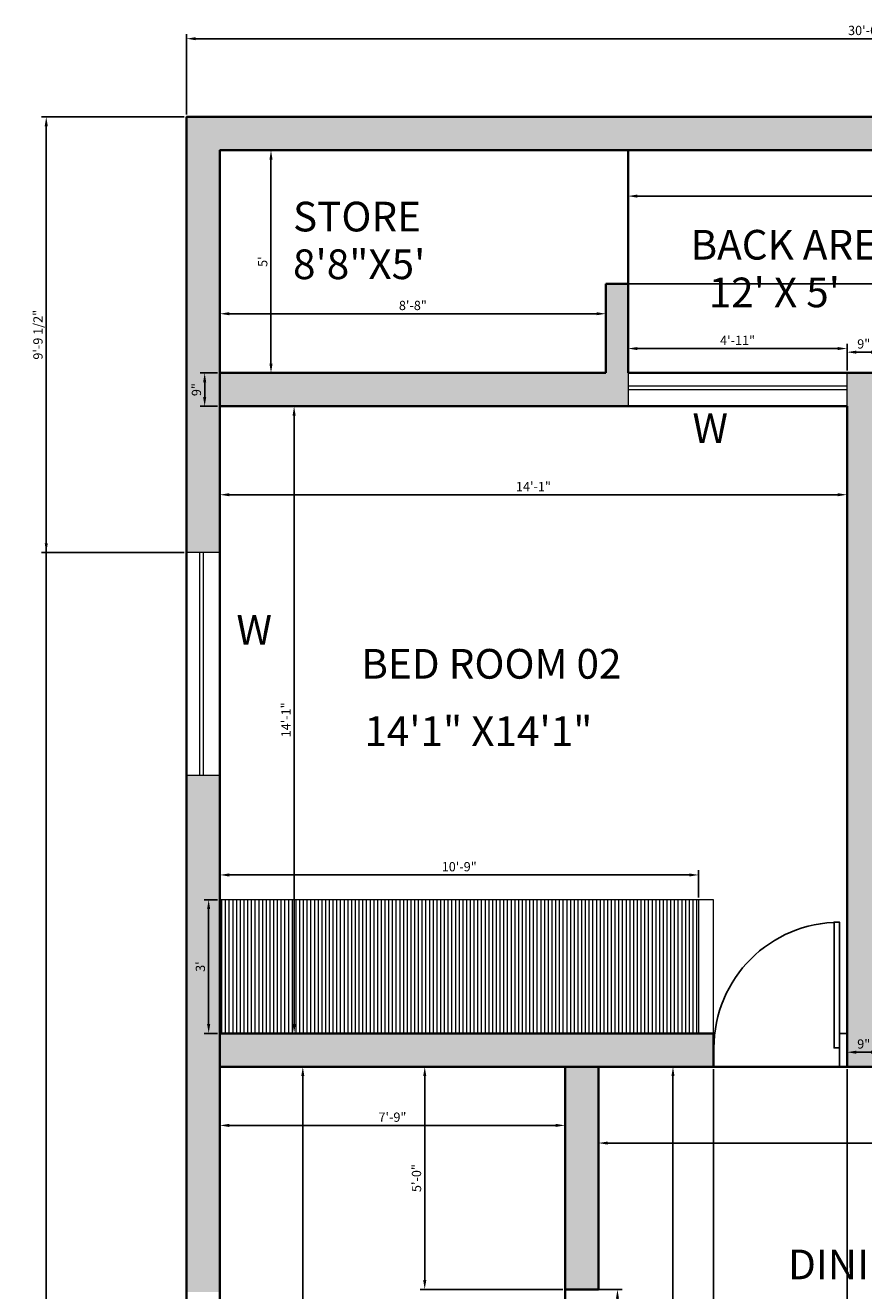
# Model space of a CAD drawing. Units: inches. Extents: x 844 to 1293, y 1224 to 2014.
# Tile 3 of 4: x 844 to 1070, y 1673 to 2014. Entities that reach past the tile are written whole.
import ezdxf

# ---------------------------------------------------------------- set-up
doc = ezdxf.new("R2010")
doc.units = ezdxf.units.IN
for name, color, linetype, lineweight in [('A-ANNO-DIMS', 2, 'Continuous', 18), ('A-ANNO-TEXT', 3, 'Continuous', 18), ('A-AREA-IDEN', 7, 'Continuous', 25), ('A-DOOR', 3, 'Continuous', 25), ('A-FLOR-PATT', 8, 'Continuous', 13), ('A-GLAZ', 4, 'Continuous', 18), ('A-WALL', 7, 'Continuous', 35), ('A-WALL-PATT', 252, 'Continuous', 13)]:
    doc.layers.add(name, color=color, linetype=linetype, lineweight=lineweight)
doc.styles.get("Standard").update_dxf_attribs({"font": 'arial.ttf'})
doc.dimstyles.new('Copy of ISO-25', dxfattribs={"dimtxt": 2.5, "dimasz": 2.5, "dimexe": 1.25, "dimexo": 0.625, "dimtad": 1, "dimlunit": 4, "dimtxsty": 'Standard', "dimcen": 2.5, "dimadec": 0, "dimazin": 0, "dimtfac": 1, "dimtmove": 0, "dimatfit": 3, "dimfxl": 1, "dimarcsym": 0})

# ---------------------------------------------------------------- blocks, each defined once
blk = doc.blocks.new('*U2')
for p, q in [((0, 0), (0, -6)), ((-40, 0), (-40, -6))]:
    blk.add_line(p, q)
blk.add_lwpolyline([(0, 0), (0, 40), (-1.75, 40), (-1.75, 0)], close=True)
blk.add_arc((0, 0), 40, 90, 180)
blk = doc.blocks.new('*D7')
at = {"layer": 'A-ANNO-DIMS', "color": 0, "lineweight": -2, "transparency": 16777216}
for p, q in [((896.46, 1910.42), (896.46, 1885.96)), ((1065.46, 1910.42), (1065.46, 1885.96)), ((898.96, 1887.21), (1062.96, 1887.21))]:
    blk.add_line(p, q, dxfattribs=at)
at = {"layer": 'A-ANNO-DIMS', "color": 0, "transparency": 16777216}
for points in [[(898.96, 1887.63), (898.96, 1886.8), (896.46, 1887.21)], [(1062.96, 1887.63), (1062.96, 1886.8), (1065.46, 1887.21)]]:
    blk.add_solid(points, dxfattribs=at)
at = {"layer": 'Defpoints', "color": 0, "transparency": 16777216}
for p in [(896.46, 1911.04), (1065.46, 1911.04), (1065.46, 1887.21)]:
    blk.add_point(p, dxfattribs=at)
at = {"layer": 'A-ANNO-DIMS', "color": 0, "transparency": 16777216, "insert": (980.96, 1889.09), "char_height": 2.5, "attachment_point": 5}
blk.add_mtext('14\'-1"', dxfattribs=at)
blk = doc.blocks.new('*D8')
at = {"layer": 'A-ANNO-DIMS', "color": 0, "lineweight": -2, "transparency": 16777216}
for p, q in [((897.09, 1911.04), (917.71, 1911.04)), ((916.46, 1908.54), (916.46, 1744.54)), ((897.09, 1742.04), (917.71, 1742.04))]:
    blk.add_line(p, q, dxfattribs=at)
at = {"layer": 'A-ANNO-DIMS', "color": 0, "transparency": 16777216}
for points in [[(916.05, 1908.54), (916.88, 1908.54), (916.46, 1911.04)], [(916.05, 1744.54), (916.88, 1744.54), (916.46, 1742.04)]]:
    blk.add_solid(points, dxfattribs=at)
at = {"layer": 'Defpoints', "color": 0, "transparency": 16777216}
for p in [(896.46, 1911.04), (896.46, 1742.04), (916.46, 1742.04)]:
    blk.add_point(p, dxfattribs=at)
at = {"layer": 'A-ANNO-DIMS', "color": 0, "transparency": 16777216, "insert": (914.58, 1826.54), "char_height": 2.5, "attachment_point": 5, "rotation": 90}
blk.add_mtext('14\'-1"', dxfattribs=at)
blk = doc.blocks.new('*D9')
at = {"layer": 'A-ANNO-DIMS', "color": 0, "lineweight": -2, "transparency": 16777216}
for p, q in [((896.46, 1920.67), (896.46, 1937.24)), ((1000.46, 1920.67), (1000.46, 1937.24)), ((898.96, 1935.99), (997.96, 1935.99))]:
    blk.add_line(p, q, dxfattribs=at)
at = {"layer": 'A-ANNO-DIMS', "color": 0, "transparency": 16777216}
for points in [[(898.96, 1936.41), (898.96, 1935.58), (896.46, 1935.99)], [(997.96, 1936.41), (997.96, 1935.58), (1000.46, 1935.99)]]:
    blk.add_solid(points, dxfattribs=at)
at = {"layer": 'Defpoints', "color": 0, "transparency": 16777216}
for p in [(1000.46, 1935.99), (896.46, 1920.04), (1000.46, 1920.04)]:
    blk.add_point(p, dxfattribs=at)
at = {"layer": 'A-ANNO-DIMS', "color": 0, "transparency": 16777216, "insert": (948.46, 1937.9), "char_height": 2.5, "attachment_point": 5}
blk.add_mtext('8\'-8"', dxfattribs=at)
blk = doc.blocks.new('*D10')
at = {"layer": 'A-ANNO-DIMS', "color": 0, "lineweight": -2, "transparency": 16777216}
for p, q in [((897.09, 1980.04), (911.48, 1980.04)), ((910.23, 1977.54), (910.23, 1922.54)), ((897.09, 1920.04), (911.48, 1920.04))]:
    blk.add_line(p, q, dxfattribs=at)
at = {"layer": 'A-ANNO-DIMS', "color": 0, "transparency": 16777216}
for points in [[(909.81, 1977.54), (910.65, 1977.54), (910.23, 1980.04)], [(909.81, 1922.54), (910.65, 1922.54), (910.23, 1920.04)]]:
    blk.add_solid(points, dxfattribs=at)
at = {"layer": 'Defpoints', "color": 0, "transparency": 16777216}
for p in [(896.46, 1980.04), (896.46, 1920.04), (910.23, 1920.04)]:
    blk.add_point(p, dxfattribs=at)
at = {"layer": 'A-ANNO-DIMS', "color": 0, "transparency": 16777216, "insert": (908.33, 1950.04), "char_height": 2.5, "attachment_point": 5, "rotation": 90}
blk.add_mtext("5'", dxfattribs=at)
blk = doc.blocks.new('*D11')
at = {"layer": 'A-ANNO-DIMS', "color": 0, "lineweight": -2, "transparency": 16777216}
for p, q in [((1006.46, 1979.42), (1006.46, 1966.44)), ((1150.46, 1979.42), (1150.46, 1966.44)), ((1008.96, 1967.69), (1147.96, 1967.69))]:
    blk.add_line(p, q, dxfattribs=at)
at = {"layer": 'A-ANNO-DIMS', "color": 0, "transparency": 16777216}
for points in [[(1008.96, 1968.11), (1008.96, 1967.27), (1006.46, 1967.69)], [(1147.96, 1968.11), (1147.96, 1967.27), (1150.46, 1967.69)]]:
    blk.add_solid(points, dxfattribs=at)
at = {"layer": 'Defpoints', "color": 0, "transparency": 16777216}
for p in [(1006.46, 1980.04), (1150.46, 1980.04), (1150.46, 1967.69)]:
    blk.add_point(p, dxfattribs=at)
at = {"layer": 'A-ANNO-DIMS', "color": 0, "transparency": 16777216, "insert": (1078.46, 1969.57), "char_height": 2.5, "attachment_point": 5}
blk.add_mtext("12'", dxfattribs=at)
blk = doc.blocks.new('*D15')
at = {"layer": 'A-ANNO-DIMS', "color": 0, "lineweight": -2, "transparency": 16777216}
for p, q in [((896.46, 1732.42), (896.46, 1715.99)), ((989.46, 1732.42), (989.46, 1715.99)), ((898.96, 1717.24), (986.96, 1717.24))]:
    blk.add_line(p, q, dxfattribs=at)
at = {"layer": 'A-ANNO-DIMS', "color": 0, "transparency": 16777216}
for points in [[(898.96, 1717.66), (898.96, 1716.82), (896.46, 1717.24)], [(986.96, 1717.66), (986.96, 1716.82), (989.46, 1717.24)]]:
    blk.add_solid(points, dxfattribs=at)
at = {"layer": 'Defpoints', "color": 0, "transparency": 16777216}
for p in [(896.46, 1733.04), (989.46, 1733.04), (989.46, 1717.24)]:
    blk.add_point(p, dxfattribs=at)
at = {"layer": 'A-ANNO-DIMS', "color": 0, "transparency": 16777216, "insert": (942.96, 1719.14), "char_height": 2.5, "attachment_point": 5}
blk.add_mtext('7\'-9"', dxfattribs=at)
blk = doc.blocks.new('*D16')
at = {"layer": 'A-ANNO-DIMS', "color": 0, "lineweight": -2, "transparency": 16777216}
for p, q in [((897.09, 1733.04), (920.05, 1733.04)), ((918.8, 1730.54), (918.8, 1565.54)), ((897.09, 1563.04), (920.05, 1563.04))]:
    blk.add_line(p, q, dxfattribs=at)
at = {"layer": 'A-ANNO-DIMS', "color": 0, "transparency": 16777216}
for points in [[(918.39, 1730.54), (919.22, 1730.54), (918.8, 1733.04)], [(918.39, 1565.54), (919.22, 1565.54), (918.8, 1563.04)]]:
    blk.add_solid(points, dxfattribs=at)
at = {"layer": 'Defpoints', "color": 0, "transparency": 16777216}
for p in [(896.46, 1733.04), (896.46, 1563.04), (918.8, 1563.04)]:
    blk.add_point(p, dxfattribs=at)
at = {"layer": 'A-ANNO-DIMS', "color": 0, "transparency": 16777216, "insert": (916.92, 1648.04), "char_height": 2.5, "attachment_point": 5, "rotation": 90}
blk.add_mtext('14\'-2"', dxfattribs=at)
blk = doc.blocks.new('*D18')
at = {"layer": 'A-ANNO-DIMS', "color": 0, "lineweight": -2, "transparency": 16777216}
for p, q in [((998.46, 1732.42), (998.46, 1711.23)), ((1244.46, 1732.42), (1244.46, 1711.23)), ((1000.96, 1712.48), (1241.96, 1712.48))]:
    blk.add_line(p, q, dxfattribs=at)
at = {"layer": 'A-ANNO-DIMS', "color": 0, "transparency": 16777216}
for points in [[(1000.96, 1712.89), (1000.96, 1712.06), (998.46, 1712.48)], [(1241.96, 1712.89), (1241.96, 1712.06), (1244.46, 1712.48)]]:
    blk.add_solid(points, dxfattribs=at)
at = {"layer": 'Defpoints', "color": 0, "transparency": 16777216}
for p in [(998.46, 1733.04), (1244.46, 1733.04), (1244.46, 1712.48)]:
    blk.add_point(p, dxfattribs=at)
at = {"layer": 'A-ANNO-DIMS', "color": 0, "transparency": 16777216, "insert": (1121.46, 1714.38), "char_height": 2.5, "attachment_point": 5}
blk.add_mtext('20\'-6"', dxfattribs=at)
blk = doc.blocks.new('*D19')
at = {"layer": 'A-ANNO-DIMS', "color": 0, "lineweight": -2, "transparency": 16777216}
for p, q in [((999.09, 1733.04), (1019.81, 1733.04)), ((1018.56, 1730.54), (1018.56, 1556.54)), ((999.09, 1554.04), (1019.81, 1554.04))]:
    blk.add_line(p, q, dxfattribs=at)
at = {"layer": 'A-ANNO-DIMS', "color": 0, "transparency": 16777216}
for points in [[(1018.14, 1730.54), (1018.97, 1730.54), (1018.56, 1733.04)], [(1018.14, 1556.54), (1018.97, 1556.54), (1018.56, 1554.04)]]:
    blk.add_solid(points, dxfattribs=at)
at = {"layer": 'Defpoints', "color": 0, "transparency": 16777216}
for p in [(998.46, 1733.04), (998.46, 1554.04), (1018.56, 1554.04)]:
    blk.add_point(p, dxfattribs=at)
at = {"layer": 'A-ANNO-DIMS', "color": 0, "transparency": 16777216, "insert": (1016.68, 1643.54), "char_height": 2.5, "attachment_point": 5, "rotation": 90}
blk.add_mtext('14\'-11"', dxfattribs=at)
blk = doc.blocks.new('*D26')
at = {"layer": 'A-ANNO-DIMS', "color": 0, "lineweight": -2, "transparency": 16777216}
for p, q in [((1006.46, 1920.67), (1006.46, 1927.86)), ((1065.46, 1920.67), (1065.46, 1927.86)), ((1008.96, 1926.61), (1062.96, 1926.61))]:
    blk.add_line(p, q, dxfattribs=at)
at = {"layer": 'A-ANNO-DIMS', "color": 0, "transparency": 16777216}
for points in [[(1008.96, 1927.02), (1008.96, 1926.19), (1006.46, 1926.61)], [(1062.96, 1927.02), (1062.96, 1926.19), (1065.46, 1926.61)]]:
    blk.add_solid(points, dxfattribs=at)
at = {"layer": 'Defpoints', "color": 0, "transparency": 16777216}
for p in [(1065.46, 1926.61), (1006.46, 1920.04), (1065.46, 1920.04)]:
    blk.add_point(p, dxfattribs=at)
at = {"layer": 'A-ANNO-DIMS', "color": 0, "transparency": 16777216, "insert": (1035.96, 1928.49), "char_height": 2.5, "attachment_point": 5}
blk.add_mtext('4\'-11"', dxfattribs=at)
blk = doc.blocks.new('*D30')
at = {"layer": 'A-ANNO-DIMS', "color": 0, "lineweight": -2, "transparency": 16777216}
for p, q in [((887.46, 1989.67), (887.46, 2011.37)), ((889.96, 2010.12), (1250.96, 2010.12)), ((1253.46, 1989.67), (1253.46, 2011.37))]:
    blk.add_line(p, q, dxfattribs=at)
at = {"layer": 'A-ANNO-DIMS', "color": 0, "transparency": 16777216}
for points in [[(889.96, 2010.54), (889.96, 2009.71), (887.46, 2010.12)], [(1250.96, 2010.54), (1250.96, 2009.71), (1253.46, 2010.12)]]:
    blk.add_solid(points, dxfattribs=at)
at = {"layer": 'Defpoints', "color": 0, "transparency": 16777216}
for p in [(1253.46, 2010.12), (887.46, 1989.04), (1253.46, 1989.04)]:
    blk.add_point(p, dxfattribs=at)
at = {"layer": 'A-ANNO-DIMS', "color": 0, "transparency": 16777216, "insert": (1070.46, 2012.02), "char_height": 2.5, "attachment_point": 5}
blk.add_mtext('30\'-6"', dxfattribs=at)
blk = doc.blocks.new('*D34')
at = {"layer": 'A-ANNO-DIMS', "color": 0, "lineweight": -2, "transparency": 16777216}
for p, q in [((1065.46, 1920.67), (1065.46, 1926.88)), ((1074.46, 1920.67), (1074.46, 1926.88)), ((1067.96, 1925.63), (1071.96, 1925.63))]:
    blk.add_line(p, q, dxfattribs=at)
at = {"layer": 'A-ANNO-DIMS', "color": 0, "transparency": 16777216}
for points in [[(1067.96, 1926.05), (1067.96, 1925.22), (1065.46, 1925.63)], [(1071.96, 1926.05), (1071.96, 1925.22), (1074.46, 1925.63)]]:
    blk.add_solid(points, dxfattribs=at)
at = {"layer": 'Defpoints', "color": 0, "transparency": 16777216}
for p in [(1074.46, 1925.63), (1065.46, 1920.04), (1074.46, 1920.04)]:
    blk.add_point(p, dxfattribs=at)
at = {"layer": 'A-ANNO-DIMS', "color": 0, "transparency": 16777216, "insert": (1069.96, 1927.53), "char_height": 2.5, "attachment_point": 5}
blk.add_mtext('9"', dxfattribs=at)
blk = doc.blocks.new('*D35')
at = {"layer": 'A-ANNO-DIMS', "color": 0, "lineweight": -2, "transparency": 16777216}
for p, q in [((895.84, 1920.04), (891.11, 1920.04)), ((892.36, 1913.54), (892.36, 1917.54)), ((895.84, 1911.04), (891.11, 1911.04))]:
    blk.add_line(p, q, dxfattribs=at)
at = {"layer": 'A-ANNO-DIMS', "color": 0, "transparency": 16777216}
for points in [[(891.94, 1917.54), (892.77, 1917.54), (892.36, 1920.04)], [(891.94, 1913.54), (892.77, 1913.54), (892.36, 1911.04)]]:
    blk.add_solid(points, dxfattribs=at)
at = {"layer": 'Defpoints', "color": 0, "transparency": 16777216}
for p in [(892.36, 1920.04), (896.46, 1920.04), (896.46, 1911.04)]:
    blk.add_point(p, dxfattribs=at)
at = {"layer": 'A-ANNO-DIMS', "color": 0, "transparency": 16777216, "insert": (890.45, 1915.54), "char_height": 2.5, "attachment_point": 5, "rotation": 90}
blk.add_mtext('9"', dxfattribs=at)
blk = doc.blocks.new('*D36')
at = {"layer": 'A-ANNO-DIMS', "color": 0, "lineweight": -2, "transparency": 16777216}
for p, q in [((1065.46, 1733.67), (1065.46, 1738.21)), ((1067.96, 1736.96), (1071.96, 1736.96)), ((1074.46, 1733.67), (1074.46, 1738.21))]:
    blk.add_line(p, q, dxfattribs=at)
at = {"layer": 'A-ANNO-DIMS', "color": 0, "transparency": 16777216}
for points in [[(1067.96, 1737.38), (1067.96, 1736.54), (1065.46, 1736.96)], [(1071.96, 1737.38), (1071.96, 1736.54), (1074.46, 1736.96)]]:
    blk.add_solid(points, dxfattribs=at)
at = {"layer": 'Defpoints', "color": 0, "transparency": 16777216}
for p in [(1074.46, 1736.96), (1065.46, 1733.04), (1074.46, 1733.04)]:
    blk.add_point(p, dxfattribs=at)
at = {"layer": 'A-ANNO-DIMS', "color": 0, "transparency": 16777216, "insert": (1069.96, 1738.86), "char_height": 2.5, "attachment_point": 5}
blk.add_mtext('9"', dxfattribs=at)
blk = doc.blocks.new('*D39')
at = {"layer": 'A-ANNO-DIMS', "color": 0, "lineweight": -2, "transparency": 16777216}
for p, q in [((895.84, 1778.04), (892.18, 1778.04)), ((893.43, 1775.54), (893.43, 1744.54)), ((895.84, 1742.04), (892.18, 1742.04))]:
    blk.add_line(p, q, dxfattribs=at)
at = {"layer": 'A-ANNO-DIMS', "color": 0, "transparency": 16777216}
for points in [[(893.01, 1775.54), (893.84, 1775.54), (893.43, 1778.04)], [(893.01, 1744.54), (893.84, 1744.54), (893.43, 1742.04)]]:
    blk.add_solid(points, dxfattribs=at)
at = {"layer": 'Defpoints', "color": 0, "transparency": 16777216}
for p in [(896.46, 1778.04), (893.43, 1742.04), (896.46, 1742.04)]:
    blk.add_point(p, dxfattribs=at)
at = {"layer": 'A-ANNO-DIMS', "color": 0, "transparency": 16777216, "insert": (891.52, 1760.04), "char_height": 2.5, "attachment_point": 5, "rotation": 90}
blk.add_mtext("3'", dxfattribs=at)
blk = doc.blocks.new('*D40')
at = {"layer": 'A-ANNO-DIMS', "color": 0, "lineweight": -2, "transparency": 16777216}
for p, q in [((896.46, 1778.67), (896.46, 1785.99)), ((898.96, 1784.74), (1022.96, 1784.74)), ((1025.46, 1778.67), (1025.46, 1785.99))]:
    blk.add_line(p, q, dxfattribs=at)
at = {"layer": 'A-ANNO-DIMS', "color": 0, "transparency": 16777216}
for points in [[(898.96, 1785.15), (898.96, 1784.32), (896.46, 1784.74)], [(1022.96, 1785.15), (1022.96, 1784.32), (1025.46, 1784.74)]]:
    blk.add_solid(points, dxfattribs=at)
at = {"layer": 'Defpoints', "color": 0, "transparency": 16777216}
for p in [(1025.46, 1784.74), (896.46, 1778.04), (1025.46, 1778.04)]:
    blk.add_point(p, dxfattribs=at)
at = {"layer": 'A-ANNO-DIMS', "color": 0, "transparency": 16777216, "insert": (960.96, 1786.64), "char_height": 2.5, "attachment_point": 5}
blk.add_mtext('10\'-9"', dxfattribs=at)
blk = doc.blocks.new('*D42')
at = {"layer": 'A-ANNO-DIMS', "color": 0, "lineweight": -2, "transparency": 16777216}
for p, q in [((990.09, 1673.04), (1004.85, 1673.04)), ((1003.6, 1625.54), (1003.6, 1670.54)), ((990.09, 1623.04), (1004.85, 1623.04))]:
    blk.add_line(p, q, dxfattribs=at)
at = {"layer": 'A-ANNO-DIMS', "color": 0, "transparency": 16777216}
for points in [[(1003.19, 1670.54), (1004.02, 1670.54), (1003.6, 1673.04)], [(1003.19, 1625.54), (1004.02, 1625.54), (1003.6, 1623.04)]]:
    blk.add_solid(points, dxfattribs=at)
at = {"layer": 'Defpoints', "color": 0, "transparency": 16777216}
for p in [(989.46, 1673.04), (1003.6, 1673.04), (989.46, 1623.04)]:
    blk.add_point(p, dxfattribs=at)
at = {"layer": 'A-ANNO-DIMS', "color": 0, "transparency": 16777216, "insert": (1001.72, 1648.04), "char_height": 2.5, "attachment_point": 5, "rotation": 90}
blk.add_mtext('4\'-2"', dxfattribs=at)
blk = doc.blocks.new('WIN-GLAZ-60IN')
for p, q in [((0, 60), (0, 0)), ((1, 60), (1, 0))]:
    blk.add_line(p, q)
blk = doc.blocks.new('*D51')
at = {"layer": 'A-ANNO-DIMS', "color": 0, "lineweight": -2, "transparency": 16777216}
for p, q in [((988.84, 1733.04), (950.41, 1733.04)), ((951.66, 1675.54), (951.66, 1730.54)), ((988.84, 1673.04), (950.41, 1673.04))]:
    blk.add_line(p, q, dxfattribs=at)
at = {"layer": 'A-ANNO-DIMS', "color": 0, "transparency": 16777216}
for points in [[(951.25, 1730.54), (952.08, 1730.54), (951.66, 1733.04)], [(951.25, 1675.54), (952.08, 1675.54), (951.66, 1673.04)]]:
    blk.add_solid(points, dxfattribs=at)
at = {"layer": 'Defpoints', "color": 0, "transparency": 16777216}
for p in [(951.66, 1733.04), (989.46, 1733.04), (989.46, 1673.04)]:
    blk.add_point(p, dxfattribs=at)
at = {"layer": 'A-ANNO-DIMS', "color": 0, "transparency": 16777216, "insert": (949.76, 1703.04), "char_height": 2.5, "attachment_point": 5, "rotation": 90}
blk.add_mtext('5\'-0"', dxfattribs=at)
blk = doc.blocks.new('*D52')
at = {"layer": 'A-ANNO-DIMS', "color": 0, "lineweight": -2, "transparency": 16777216}
for p, q in [((886.84, 1989.04), (848.41, 1989.04)), ((849.66, 1265.54), (849.66, 1986.54)), ((886.84, 1263.04), (848.41, 1263.04))]:
    blk.add_line(p, q, dxfattribs=at)
at = {"layer": 'A-ANNO-DIMS', "color": 0, "transparency": 16777216}
for points in [[(849.25, 1986.54), (850.08, 1986.54), (849.66, 1989.04)], [(849.25, 1265.54), (850.08, 1265.54), (849.66, 1263.04)]]:
    blk.add_solid(points, dxfattribs=at)
at = {"layer": 'Defpoints', "color": 0, "transparency": 16777216}
for p in [(849.66, 1989.04), (887.46, 1989.04), (887.46, 1263.04)]:
    blk.add_point(p, dxfattribs=at)
at = {"layer": 'A-ANNO-DIMS', "color": 0, "transparency": 16777216, "insert": (847.76, 1626.04), "char_height": 2.5, "attachment_point": 5, "rotation": 90}
blk.add_mtext('60\'-6"', dxfattribs=at)
blk = doc.blocks.new('*D54')
at = {"layer": 'A-ANNO-DIMS', "color": 0, "lineweight": -2, "transparency": 16777216}
for p, q in [((886.84, 1989.04), (848.41, 1989.04)), ((849.66, 1874.12), (849.66, 1986.54)), ((886.84, 1871.62), (848.41, 1871.62))]:
    blk.add_line(p, q, dxfattribs=at)
at = {"layer": 'A-ANNO-DIMS', "color": 0, "transparency": 16777216}
for points in [[(849.25, 1986.54), (850.08, 1986.54), (849.66, 1989.04)], [(849.25, 1874.12), (850.08, 1874.12), (849.66, 1871.62)]]:
    blk.add_solid(points, dxfattribs=at)
at = {"layer": 'Defpoints', "color": 0, "transparency": 16777216}
for p in [(849.66, 1989.04), (887.46, 1989.04), (887.46, 1871.62)]:
    blk.add_point(p, dxfattribs=at)
at = {"layer": 'A-ANNO-DIMS', "color": 0, "transparency": 16777216, "insert": (847.75, 1930.33), "char_height": 2.5, "attachment_point": 5, "rotation": 90}
blk.add_mtext('9\'-9 1/2"', dxfattribs=at)
blk = doc.blocks.new('*D65')
at = {"layer": 'A-ANNO-DIMS', "color": 0, "lineweight": -2, "transparency": 16777216}
for p, q in [((1007.09, 1980.04), (1292.51, 1980.04)), ((1291.26, 1946.54), (1291.26, 1977.54)), ((1001.09, 1944.04), (1292.51, 1944.04))]:
    blk.add_line(p, q, dxfattribs=at)
at = {"layer": 'A-ANNO-DIMS', "color": 0, "transparency": 16777216}
for points in [[(1290.85, 1977.54), (1291.68, 1977.54), (1291.26, 1980.04)], [(1290.85, 1946.54), (1291.68, 1946.54), (1291.26, 1944.04)]]:
    blk.add_solid(points, dxfattribs=at)
at = {"layer": 'Defpoints', "color": 0, "transparency": 16777216}
for p in [(1006.46, 1980.04), (1291.26, 1980.04), (1000.46, 1944.04)]:
    blk.add_point(p, dxfattribs=at)
at = {"layer": 'A-ANNO-DIMS', "color": 0, "transparency": 16777216, "insert": (1289.36, 1962.04), "char_height": 2.5, "attachment_point": 5, "rotation": 90}
blk.add_mtext('3\'-0"', dxfattribs=at)
blk = doc.blocks.new('*D66')
at = {"layer": 'A-ANNO-DIMS', "color": 0, "lineweight": -2, "transparency": 16777216}
for p, q in [((1029.46, 1732.42), (1029.46, 1223.99)), ((1065.46, 1732.42), (1065.46, 1223.99)), ((1031.96, 1225.24), (1062.96, 1225.24))]:
    blk.add_line(p, q, dxfattribs=at)
at = {"layer": 'A-ANNO-DIMS', "color": 0, "transparency": 16777216}
for points in [[(1031.96, 1225.66), (1031.96, 1224.82), (1029.46, 1225.24)], [(1062.96, 1225.66), (1062.96, 1224.82), (1065.46, 1225.24)]]:
    blk.add_solid(points, dxfattribs=at)
at = {"layer": 'Defpoints', "color": 0, "transparency": 16777216}
for p in [(1029.46, 1733.04), (1065.46, 1733.04), (1065.46, 1225.24)]:
    blk.add_point(p, dxfattribs=at)
at = {"layer": 'A-ANNO-DIMS', "color": 0, "transparency": 16777216, "insert": (1047.46, 1227.14), "char_height": 2.5, "attachment_point": 5}
blk.add_mtext('3\'-0"', dxfattribs=at)

msp = doc.modelspace()

# ---------------------------------------------------------------- hatches: boundary and pattern name
at = {"layer": 'A-FLOR-PATT'}
h = msp.add_hatch(dxfattribs=at)
h.set_pattern_fill('ANSI31', color=256, scale=0.3149606, angle=45, style=0)
h.paths.add_polyline_path([(896.465, 1742.042), (1025.465, 1742.042), (1025.465, 1778.042), (896.465, 1778.042)])
at = {"layer": 'A-WALL-PATT'}
h = msp.add_hatch(color=256, dxfattribs=at)
h.dxf.hatch_style = 1
h.paths.add_polyline_path([(1253.465, 1989.042), (887.465, 1989.042), (887.465, 1920.042), (887.465, 1911.042), (887.465, 1871.621), (896.465, 1871.621), (896.465, 1911.042), (896.465, 1920.042), (896.465, 1980.042), (1000.465, 1980.042), (1244.465, 1980.042), (1244.465, 1968.042), (1253.465, 1968.042)])
h.paths.add_polyline_path([(1006.465, 1944.042), (1000.465, 1944.042), (1000.465, 1920.042), (896.465, 1920.042), (896.465, 1911.042), (1006.465, 1911.042), (1006.465, 1920.042)], flags=17)
h.paths.add_polyline_path([(1253.465, 1968.042), (1244.465, 1968.042), (1244.465, 1932.042), (1253.465, 1932.042)], flags=17)
h.paths.add_polyline_path([(1253.465, 1920.042), (1253.465, 1932.042), (1244.465, 1932.042), (1244.465, 1920.042), (1244.465, 1911.042), (1244.465, 1884.775), (1253.465, 1884.775), (1253.465, 1911.042)], flags=17)
h.paths.add_polyline_path([(1208.465, 1920.042), (1156.465, 1920.042), (1156.465, 1980.042), (1150.465, 1980.042), (1150.465, 1920.042), (1150.465, 1911.042), (1208.465, 1911.042)], flags=17)
h.paths.add_polyline_path([(1110.465, 1920.042), (1074.465, 1920.042), (1074.465, 1911.042), (1110.465, 1911.042)], flags=17)
h.paths.add_polyline_path([(896.465, 1811.621), (887.465, 1811.621), (887.465, 1672.343), (896.465, 1672.343), (896.465, 1733.042), (896.465, 1742.042)])
h.paths.add_polyline_path([(896.465, 1624.343), (887.465, 1624.343), (887.465, 1263.042), (1253.465, 1263.042), (1253.465, 1574.212), (1244.465, 1574.212), (1244.465, 1563.042), (1244.465, 1554.042), (1244.465, 1272.042), (1016.465, 1272.042), (1016.465, 1267.542), (896.465, 1267.542), (896.465, 1272.042), (896.465, 1554.042), (968.465, 1554.042), (989.465, 1554.042), (998.465, 1554.042), (998.465, 1623.042), (989.465, 1623.042), (989.465, 1563.042), (896.465, 1563.042)])
h.paths.add_polyline_path([(998.465, 1518.042), (994.855, 1518.042), (989.465, 1518.042), (989.465, 1497.104), (998.465, 1497.104)], flags=17)
h.paths.add_polyline_path([(998.465, 1449.104), (989.465, 1449.104), (989.465, 1391.042), (998.465, 1391.042), (1070.313, 1391.042), (1070.313, 1396.464), (1070.313, 1400.042), (998.465, 1400.042)], flags=17)
h.paths.add_polyline_path([(1112.465, 1450.531), (1106.465, 1450.531), (1106.465, 1400.042), (1106.465, 1391.042), (1112.465, 1391.042)], flags=17)
h.paths.add_polyline_path([(1112.465, 1554.042), (1112.394, 1554.042), (1112.394, 1559.602, -0.015479), (1112.465, 1561.896), (1112.465, 1563.042), (1106.465, 1563.042), (1106.465, 1554.042), (1106.465, 1510.531), (1112.465, 1510.531)], flags=17)
h.paths.add_polyline_path([(1158.465, 1623.042), (1244.465, 1623.042), (1244.465, 1632.042), (1158.465, 1632.042), (1149.465, 1632.042), (1149.465, 1599.042), (1158.465, 1599.042)])
h.paths.add_polyline_path([(1244.465, 1563.042), (1158.465, 1563.042), (1149.465, 1563.042), (1149.465, 1554.042), (1244.465, 1554.042)], flags=17)
h.paths.add_polyline_path([(1253.465, 1650.728), (1244.465, 1650.728), (1244.465, 1610.212), (1253.465, 1610.212)])
h.paths.add_polyline_path([(998.465, 1733.042), (989.465, 1733.042), (989.465, 1673.042), (998.465, 1673.042)])
h.paths.add_polyline_path([(1029.465, 1742.042), (896.465, 1742.042), (896.465, 1733.042), (989.465, 1733.042), (1029.465, 1733.042)])
h.paths.add_polyline_path([(1244.465, 1742.042), (1110.465, 1742.042), (1110.465, 1739.692, -0.0113533), (1110.5, 1738.147), (1110.5, 1733.042), (1244.465, 1733.042)])
h.paths.add_polyline_path([(1253.465, 1812.775), (1244.465, 1812.775), (1244.465, 1710.728), (1253.465, 1710.728)])
h.paths.add_polyline_path([(1074.465, 1911.042), (1074.465, 1920.042), (1065.465, 1920.042), (1065.465, 1911.042), (1065.465, 1742.042), (1065.465, 1733.042), (1074.465, 1733.042), (1074.465, 1742.042)])
h.paths.add_polyline_path([(1067.758, 1736.261), (1072.19, 1736.261), (1072.19, 1741.413), (1067.758, 1741.413)], flags=24)
h.paths.add_polyline_path([(975.783, 1886.472), (985.93, 1886.472), (985.93, 1891.624), (975.783, 1891.624)], flags=25)
h.paths.add_polyline_path([(917.205, 1821.36), (917.205, 1831.507), (912.053, 1831.507), (912.053, 1821.36)], flags=9)
h.paths.add_polyline_path([(1050.545, 1543.381), (1054.404, 1543.381), (1054.404, 1548.533), (1050.545, 1548.533)], flags=25)
h.paths.add_polyline_path([(1116.422, 1711.778), (1126.569, 1711.778), (1126.569, 1716.93), (1116.422, 1716.93)], flags=9)
h.paths.add_polyline_path([(1019.298, 1637.389), (1019.298, 1649.478), (1014.146, 1649.478), (1014.146, 1637.389)], flags=9)
h.paths.add_polyline_path([(980.864, 1534.121), (980.864, 1537.98), (975.712, 1537.98), (975.712, 1534.121)], flags=25)
h.paths.add_polyline_path([(1019.234, 1470.889), (1019.234, 1482.978), (1014.082, 1482.978), (1014.082, 1470.889)], flags=25)
h.paths.add_polyline_path([(1175.456, 1538.714), (1181.257, 1538.714), (1181.257, 1543.865), (1175.456, 1543.865)], flags=25)
h.paths.add_polyline_path([(1122.736, 1467.36), (1122.736, 1477.507), (1117.584, 1477.507), (1117.584, 1467.36)], flags=25)
h.paths.add_polyline_path([(907.276, 1556.335), (907.276, 1560.767), (902.124, 1560.767), (902.124, 1556.335)], flags=24)
h.paths.add_polyline_path([(1107.309, 1567.013), (1111.742, 1567.013), (1111.742, 1572.165), (1107.309, 1572.165)], flags=25)
h.paths.add_polyline_path([(955.783, 1784.038), (965.93, 1784.038), (965.93, 1789.19), (955.783, 1789.19)], flags=9)
h.paths.add_polyline_path([(1004.344, 1643.999), (1004.344, 1652.203), (999.192, 1652.203), (999.192, 1643.999)], flags=9)
h.paths.add_polyline_path([(973.263, 1534.121), (973.263, 1537.98), (968.111, 1537.98), (968.111, 1534.121)], flags=25)
h.paths.add_polyline_path([(1047.536, 1660.728), (1114.78, 1660.728), (1114.78, 1672.982), (1047.536, 1672.982)], flags=9)
h.paths.add_polyline_path([(1047.509, 1673.552), (1128.636, 1673.552), (1128.636, 1685.969), (1047.509, 1685.969)], flags=9)
h.paths.add_polyline_path([(999.825, 1474.75), (1014.374, 1474.75), (1014.374, 1486.75), (999.825, 1486.75)], flags=25)
h.paths.add_polyline_path([(1085.974, 1473.689), (1100.523, 1473.689), (1100.523, 1485.689), (1085.974, 1485.689)], flags=25)
h.paths.add_polyline_path([(898.914, 1844.786), (913.462, 1844.786), (913.462, 1856.786), (898.914, 1856.786)], flags=9)
h.paths.add_polyline_path([(1021.801, 1899.15), (1036.35, 1899.15), (1036.35, 1911.15), (1021.801, 1911.15)], flags=25)
h.paths.add_polyline_path([(933.371, 1817.465), (997.445, 1817.465), (997.445, 1829.522), (933.371, 1829.522)], flags=9)
h.paths.add_polyline_path([(912.536, 1375.627), (960.277, 1375.627), (960.277, 1387.881), (912.536, 1387.881)], flags=25)
h.paths.add_polyline_path([(908.723, 1393.944), (979.923, 1393.944), (979.923, 1406.361), (908.723, 1406.361)], flags=25)
h.paths.add_polyline_path([(907.199, 1415.111), (926.792, 1415.111), (926.792, 1427.316), (907.199, 1427.316)], flags=25)
h.paths.add_polyline_path([(1130.034, 1467.266), (1180.017, 1467.266), (1180.017, 1479.52), (1130.034, 1479.52)], flags=25)
h.paths.add_polyline_path([(1130.007, 1480.09), (1210.517, 1480.09), (1210.517, 1492.508), (1130.007, 1492.508)], flags=25)
h.paths.add_polyline_path([(918.552, 1280.947), (1012.38, 1280.947), (1012.38, 1293.356), (918.552, 1293.356)], flags=25)
h.paths.add_polyline_path([(1074.912, 1322.783), (1119.613, 1322.783), (1119.613, 1334.988), (1074.912, 1334.988)], flags=25)
h.paths.add_polyline_path([(994.568, 1321.709), (1075.078, 1321.709), (1075.078, 1334.127), (994.568, 1334.127)], flags=25)
h.paths.add_polyline_path([(932.502, 1835.432), (1188.778, 1835.432), (1188.778, 1847.849), (932.502, 1847.849)], flags=9)

# ---------------------------------------------------------------- linework, layer by layer
at = {"layer": 'A-DOOR'}
for p, q in [((1063.465, 1733.042), (1063.465, 1742.042)), ((1063.465, 1742.042), (1065.465, 1742.042)), ((1065.465, 1733.042), (1063.465, 1733.042))]:
    msp.add_line(p, q, dxfattribs=at)
at = {"layer": 'A-FLOR-PATT'}
for p, q in [((1025.465, 1778.042), (896.465, 1778.042)), ((1029.465, 1778.042), (1025.465, 1778.042)), ((1025.465, 1778.042), (1025.465, 1742.042)), ((1029.465, 1742.042), (1029.465, 1778.042))]:
    msp.add_line(p, q, dxfattribs=at)
at = {"layer": 'A-GLAZ'}
for p, q in [((1006.465, 1920.042), (1006.465, 1911.042)), ((1065.465, 1911.042), (1065.465, 1920.042)), ((1006.465, 1916.542), (1065.465, 1916.542)), ((1006.465, 1915.542), (1065.465, 1915.542)), ((896.465, 1871.621), (887.465, 1871.621)), ((887.465, 1871.621), (887.465, 1811.621)), ((887.465, 1811.621), (896.465, 1811.621))]:
    msp.add_line(p, q, dxfattribs=at)
at = {"layer": 'A-WALL'}
for p, q in [((896.465, 1980.042), (1000.465, 1980.042)), ((1006.465, 1920.042), (1006.465, 1980.042)), ((1000.465, 1944.042), (1000.465, 1920.042)), ((1000.465, 1944.042), (1006.465, 1944.042)), ((887.465, 1920.042), (887.465, 1911.042)), ((1000.465, 1920.042), (896.465, 1920.042)), ((896.465, 1920.042), (896.465, 1911.042)), ((1006.465, 1920.042), (1144.465, 1920.042)), ((1006.465, 1920.042), (1074.465, 1920.042)), ((896.465, 1911.042), (1000.465, 1911.042)), ((896.465, 1911.042), (1065.465, 1911.042)), ((896.465, 1911.042), (896.465, 1871.621)), ((971.051, 1911.042), (941.051, 1911.042)), ((1000.465, 1911.042), (1065.465, 1911.042)), ((1000.465, 1911.042), (1006.465, 1911.042)), ((1065.465, 1911.042), (1065.465, 1742.042)), ((1029.465, 1742.042), (896.465, 1742.042)), ((896.465, 1742.042), (896.465, 1733.042)), ((1029.465, 1733.042), (1029.465, 1742.042)), ((1065.465, 1742.042), (1065.465, 1733.042)), ((896.465, 1733.042), (1029.465, 1733.042)), ((896.465, 1733.042), (989.465, 1733.042)), ((896.465, 1733.042), (896.465, 1672.343)), ((989.465, 1733.042), (989.465, 1673.042)), ((989.465, 1733.042), (989.465, 1673.042)), ((998.465, 1673.042), (998.465, 1733.042)), ((1029.595, 1733.042), (1244.465, 1733.042)), ((989.465, 1673.042), (998.465, 1673.042)), ((989.465, 1673.042), (989.465, 1623.042))]:
    msp.add_line(p, q, dxfattribs=at)
for points in [[(1253.465, 1920.042), (1253.465, 1989.042), (887.465, 1989.042), (887.465, 1920.042)], [(1244.465, 1920.042), (1244.465, 1980.042), (896.465, 1980.042), (896.465, 1920.042)], [(887.465, 1911.042), (887.465, 1263.042), (1253.465, 1263.042), (1253.465, 1911.042)], [(896.465, 1911.042), (896.465, 1563.042)]]:
    msp.add_lwpolyline(points, dxfattribs=at)

# ---------------------------------------------------------------- block references
at = {"layer": 'A-DOOR', "xscale": 0.846739657943228, "yscale": 0.846739657943228, "zscale": 0.846739657943228}
msp.add_blockref('*U2', (1063.465, 1738.122), dxfattribs=at)
at = {"layer": 'A-GLAZ'}
msp.add_blockref('WIN-GLAZ-60IN', (890.965, 1811.621), dxfattribs=at)

# ---------------------------------------------------------------- texts
at = {"layer": 'A-ANNO-TEXT'}
for p in [(1023.801, 1901.15), (900.914, 1846.786)]:
    msp.add_text('W', height=8, dxfattribs=at).set_placement(p)
at = {"layer": 'A-AREA-IDEN'}
for s, p in [('STORE', (916.162, 1958.174)), ('BACK AREA', (1023.293, 1950.587)), ('8\'8"X5\'', (916.162, 1945.322)), ("  12' X 5'", (1023.293, 1937.736)), ('BED ROOM 02                                BED ROOM 01', (934.572, 1837.638)), ('14\'1" X14\'1"', (935.381, 1819.48)), ('DINING ROOM', (1049.578, 1675.758))]:
    msp.add_text(s, height=8, dxfattribs=at).set_placement(p)

# ---------------------------------------------------------------- dimensions: what is measured, and where the dimension line sits
at = {"layer": 'A-ANNO-DIMS'}
for base, p1, p2, override, picture, middle in [((1253.465, 2010.122), (887.465, 1989.042), (1253.465, 1989.042), {"dimclrd": 0, "dimclre": 0, "dimclrt": 0}, '*D30', (1070.465, 2012.024)), ((1150.465, 1967.69), (1006.465, 1980.042), (1150.465, 1980.042), {"dimclrd": 0, "dimclre": 0, "dimclrt": 0}, '*D11', (1078.465, 1969.57)), ((1000.465, 1935.994), (896.465, 1920.042), (1000.465, 1920.042), {"dimclrd": 0, "dimclre": 0, "dimclrt": 0}, '*D9', (948.465, 1937.895)), ((1065.465, 1926.608), (1006.465, 1920.042), (1065.465, 1920.042), {"dimclrd": 0, "dimclre": 0, "dimclrt": 0}, '*D26', (1035.965, 1928.488)), ((1074.465, 1925.633), (1065.465, 1920.042), (1074.465, 1920.042), {"dimclrd": 0, "dimclre": 0, "dimclrt": 0}, '*D34', (1069.965, 1927.534)), ((1065.465, 1887.212), (896.465, 1911.042), (1065.465, 1911.042), {"dimclrd": 0, "dimclre": 0, "dimclrt": 0}, '*D7', (980.965, 1889.092)), ((1025.465, 1784.735), (896.465, 1778.042), (1025.465, 1778.042), {"dimclrd": 0, "dimclre": 0, "dimclrt": 0}, '*D40', (960.965, 1786.637)), ((1074.465, 1736.959), (1065.465, 1733.042), (1074.465, 1733.042), {"dimclrd": 0, "dimclre": 0, "dimclrt": 0}, '*D36', (1069.965, 1738.86)), ((989.465, 1717.241), (896.465, 1733.042), (989.465, 1733.042), {"dimclrd": 0, "dimclre": 0, "dimclrt": 0}, '*D15', (942.965, 1719.143)), ((1244.465, 1712.476), (998.465, 1733.042), (1244.465, 1733.042), {"dimclrd": 0, "dimclre": 0, "dimclrt": 0}, '*D18', (1121.465, 1714.377)), ((1065.465, 1225.242), (1029.465, 1733.042), (1065.465, 1733.042), {"dimdec": 1, "dimlfac": 1, "dimrnd": 0, "dimzin": 1, "dimdsep": 46, "dimlunit": 4, "dimfrac": 2}, '*D66', (1047.465, 1227.144))]:
    dim = msp.add_linear_dim(base=base, p1=p1, p2=p2, dimstyle='Copy of ISO-25', override=override, dxfattribs=at)
    dim.commit()
    dim.dimension.update_dxf_attribs({"geometry": picture, "text_midpoint": middle})
for base, p1, p2, override, picture, middle in [((849.665, 1989.042), (887.465, 1871.621), (887.465, 1989.042), {"dimdec": 1, "dimlfac": 1, "dimrnd": 0, "dimzin": 1, "dimdsep": 46, "dimlunit": 4, "dimfrac": 2}, '*D54', (847.747, 1930.331)), ((849.665, 1989.042), (887.465, 1263.042), (887.465, 1989.042), {"dimdec": 1, "dimlfac": 1, "dimrnd": 0, "dimzin": 1, "dimdsep": 46, "dimlunit": 4, "dimfrac": 2}, '*D52', (847.763, 1626.042)), ((910.23, 1920.042), (896.465, 1980.042), (896.465, 1920.042), {"dimclrd": 0, "dimclre": 0, "dimclrt": 0}, '*D10', (908.334, 1950.042)), ((1291.265, 1980.042), (1000.465, 1944.042), (1006.465, 1980.042), {"dimdec": 1, "dimlfac": 1, "dimrnd": 0, "dimzin": 1, "dimdsep": 46, "dimlunit": 4, "dimfrac": 2}, '*D65', (1289.363, 1962.042)), ((892.355, 1920.042), (896.465, 1911.042), (896.465, 1920.042), {"dimclrd": 0, "dimclre": 0, "dimclrt": 0}, '*D35', (890.454, 1915.542)), ((916.465, 1742.042), (896.465, 1911.042), (896.465, 1742.042), {"dimclrd": 0, "dimclre": 0, "dimclrt": 0}, '*D8', (914.585, 1826.542)), ((893.427, 1742.042), (896.465, 1778.042), (896.465, 1742.042), {"dimclrd": 0, "dimclre": 0, "dimclrt": 0}, '*D39', (891.525, 1760.042)), ((918.805, 1563.042), (896.465, 1733.042), (896.465, 1563.042), {"dimclrd": 0, "dimclre": 0, "dimclrt": 0}, '*D16', (916.925, 1648.042)), ((951.665, 1733.042), (989.465, 1673.042), (989.465, 1733.042), {"dimdec": 1, "dimlfac": 1, "dimrnd": 0, "dimzin": 1, "dimdsep": 46, "dimlunit": 4, "dimfrac": 2}, '*D51', (949.763, 1703.042)), ((1018.558, 1554.042), (998.465, 1733.042), (998.465, 1554.042), {"dimclrd": 0, "dimclre": 0, "dimclrt": 0}, '*D19', (1016.678, 1643.542)), ((1003.604, 1673.042), (989.465, 1623.042), (989.465, 1673.042), {"dimclrd": 0, "dimclre": 0, "dimclrt": 0}, '*D42', (1001.724, 1648.042))]:
    dim = msp.add_linear_dim(base=base, p1=p1, p2=p2, angle=90, dimstyle='Copy of ISO-25', override=override, dxfattribs=at)
    dim.commit()
    dim.dimension.update_dxf_attribs({"geometry": picture, "text_midpoint": middle})

doc.saveas('drawing.dxf')
